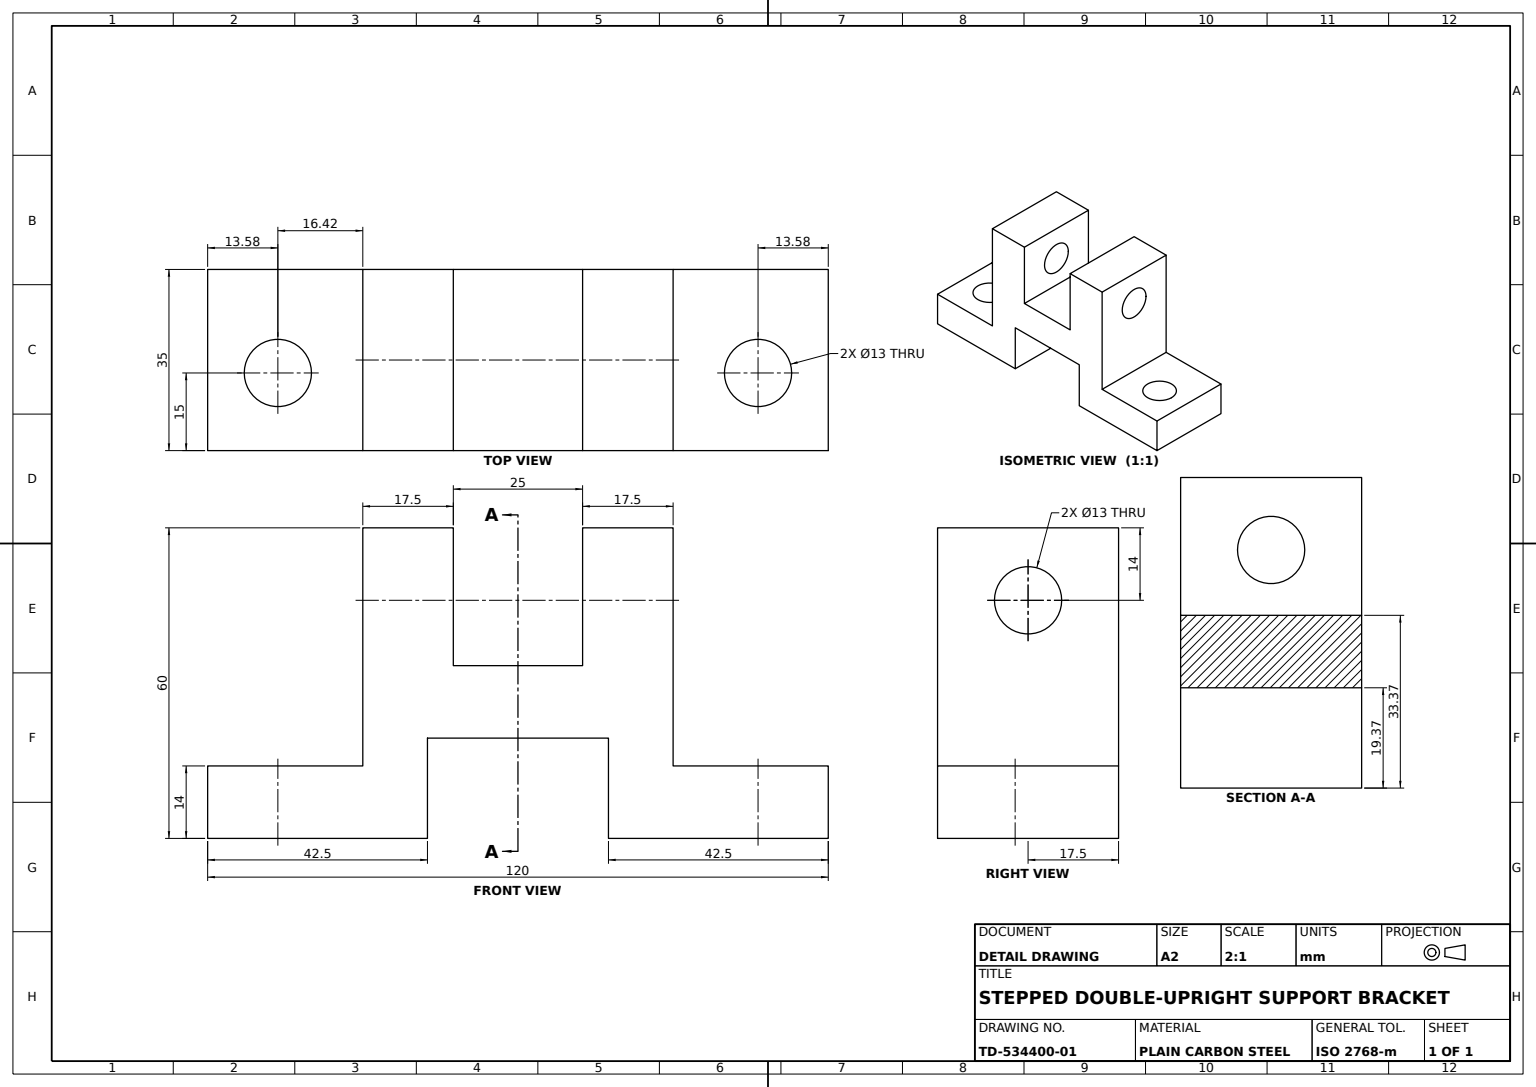
SolidWorks part; units mm, degrees
material "Plain Carbon Steel"
ref_plane "Front Plane" through (0, 0, 0) normal (0, 0, 1) x (1, 0, 0)
ref_plane "Top Plane" through (0, 0, 0) normal (0, 1, 0) x (1, 0, 0)
ref_plane "Right Plane" through (0, 0, 0) normal (1, 0, 0) x (0, 0, -1)
sketch "Fork Profile Sketch" plane through (0, 0, 0) normal (0, 0, 1) x (1, 0, 0)
  line L0 (0, 40.6254) -> (0, -38.1418) construction
  line L1 (0, 0) -> (17.5, 0)
  line L2 (17.5, 0) -> (17.5, -19.3746)
  line L3 (17.5, -19.3746) -> (60, -19.3746)
  line L4 (60, -19.3746) -> (60, -5.3746)
  line L5 (60, -5.3746) -> (30, -5.3746)
  line L6 (30, -5.3746) -> (30, 40.6254)
  line L7 (30, 40.6254) -> (12.5, 40.6254)
  line L8 (12.5, 40.6254) -> (12.5, 14)
  line L9 (12.5, 14) -> (-12.5, 14)
  line L10 (0, 0) -> (-17.5, 0)
  line L11 (-12.5, 40.6254) -> (-12.5, 14)
  line L12 (-30, 40.6254) -> (-12.5, 40.6254)
  line L13 (-30, -5.3746) -> (-30, 40.6254)
  line L14 (-60, -5.3746) -> (-30, -5.3746)
  line L15 (-60, -19.3746) -> (-60, -5.3746)
  line L16 (-17.5, -19.3746) -> (-60, -19.3746)
  line L17 (-17.5, 0) -> (-17.5, -19.3746)
  point P2 (8.75, 0)
  point P16 (0, 14)
  dimension "D1" = 17.5
  dimension "D2" = 120
  dimension "D3" = 14
  dimension "D4" = 60
  dimension "D5" = 60
  dimension "D6" = 25
  dimension "D7" = 14
  dimension "D8" = 19.3746
extrude "Fork Body" add sketch "Fork Profile Sketch" along normal blind 35
sketch "Lug Cross Hole Sketch" plane through (-30, 0, 0) normal (-1, 0, 0) x (0, 0, 1)
  line L0 (35, 40.6254) -> (0, 40.6254) construction
  line L1 (0, 40.6254) -> (0, -5.3746) construction
  circle A0 centre (17.5, 26.6254) radius 6.5
  dimension "D1" = 13
  dimension "D2" = 14
  dimension "D3" = 17.5
extrude "Lug Cross Hole Ø13" cut sketch "Lug Cross Hole Sketch" against normal through all
sketch "Base Mounting Holes Sketch" plane through (0, -5.3746, 0) normal (0, 1, 0) x (1, 0, 0)
  line L0 (60, -35) -> (30, -35) construction
  line L1 (0, -19.25) -> (0, 19.25) construction
  line L2 (30, -35) -> (30, 0) construction
  circle A0 centre (46.4239, -20) radius 6.5
  circle A1 centre (-46.4239, -20) radius 6.5
  dimension "D2" = 13
  dimension "D1" = 15
  dimension "D3" = 16.4239
extrude "Base Mounting Holes 2xØ13" cut sketch "Base Mounting Holes Sketch" against normal through all
